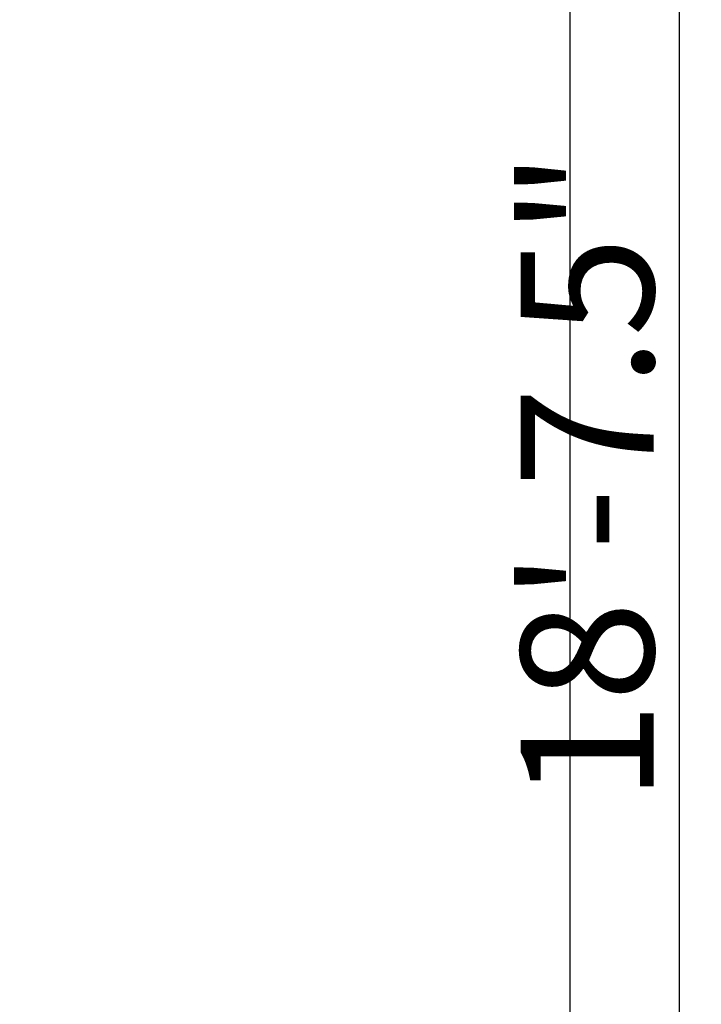
# Model space of a CAD drawing. Units: inches. Extents: x 2083 to 3317, y 1141 to 2115.
# Tile 245 of 256: x 3130 to 3191, y 1327 to 1416. Entities that reach past the tile are written whole.
import ezdxf

# ---------------------------------------------------------------- set-up
doc = ezdxf.new("R2010")
doc.units = ezdxf.units.IN
doc.layers.add('A-ANNO-DIMS', color=2, linetype='Continuous', lineweight=18)
doc.styles.get("Standard").update_dxf_attribs({"font": 'arial.ttf'})
doc.dimstyles.new('ISO-25', dxfattribs={"dimtxt": 12, "dimasz": 12, "dimexe": 1.25, "dimexo": 0.625, "dimtad": 1, "dimlunit": 3, "dimtxsty": 'Standard', "dimcen": 2.5, "dimadec": 0, "dimazin": 0, "dimtfac": 1, "dimtmove": 0, "dimatfit": 3, "dimfxl": 1, "dimarcsym": 0})

# ---------------------------------------------------------------- blocks, each defined once
blk = doc.blocks.new('*D9')
at = {"layer": 'A-ANNO-DIMS', "color": 0, "lineweight": -2, "transparency": 16777216}
for p, q in [((3127.585, 1486.761), (3190.403, 1486.761)), ((3189.153, 1474.761), (3189.153, 1275.261)), ((3127.585, 1263.261), (3190.403, 1263.261))]:
    blk.add_line(p, q, dxfattribs=at)
at = {"layer": 'A-ANNO-DIMS', "color": 0, "transparency": 16777216}
for points in [[(3187.153, 1474.761), (3191.153, 1474.761), (3189.153, 1486.761)], [(3187.153, 1275.261), (3191.153, 1275.261), (3189.153, 1263.261)]]:
    blk.add_solid(points, dxfattribs=at)
at = {"layer": 'Defpoints', "color": 0, "transparency": 16777216}
for p in [(3126.96, 1486.761), (3126.96, 1263.261), (3189.153, 1263.261)]:
    blk.add_point(p, dxfattribs=at)
at = {"layer": 'A-ANNO-DIMS', "color": 0, "transparency": 16777216, "insert": (3182.401, 1375.011), "char_height": 12, "attachment_point": 5, "rotation": 90}
blk.add_mtext('18\'-7.5"', dxfattribs=at)
blk = doc.blocks.new('*D35')
at = {"layer": 'A-ANNO-DIMS', "color": 0, "lineweight": -2, "transparency": 16777216}
for p, q in [((3127.585, 2020.761), (3180.56, 2020.761)), ((3179.31, 1275.261), (3179.31, 2008.761)), ((3127.585, 1263.261), (3180.56, 1263.261))]:
    blk.add_line(p, q, dxfattribs=at)
at = {"layer": 'A-ANNO-DIMS', "color": 0, "transparency": 16777216}
for points in [[(3177.31, 2008.761), (3181.31, 2008.761), (3179.31, 2020.761)], [(3177.31, 1275.261), (3181.31, 1275.261), (3179.31, 1263.261)]]:
    blk.add_solid(points, dxfattribs=at)
at = {"layer": 'Defpoints', "color": 0, "transparency": 16777216}
for p in [(3126.96, 2020.761), (3179.31, 2020.761), (3126.96, 1263.261)]:
    blk.add_point(p, dxfattribs=at)
at = {"layer": 'A-ANNO-DIMS', "color": 0, "transparency": 16777216, "insert": (3172.476, 1642.011), "char_height": 12, "attachment_point": 5, "rotation": 90}
blk.add_mtext('63\'-1 1/2"', dxfattribs=at)

msp = doc.modelspace()

# ---------------------------------------------------------------- dimensions: what is measured, and where the dimension line sits
at = {"layer": 'A-ANNO-DIMS'}
for base, p1, p2, override, picture, middle in [((3179.31, 2020.761), (3126.96, 1263.261), (3126.96, 2020.761), {"dimdec": 1, "dimlfac": 1, "dimrnd": 0, "dimzin": 1, "dimdsep": 46, "dimlunit": 4, "dimfrac": 2}, '*D35', (3172.476, 1642.011)), ((3189.153, 1263.261), (3126.96, 1486.761), (3126.96, 1263.261), {"dimclrd": 0, "dimclre": 0, "dimclrt": 0}, '*D9', (3182.401, 1375.011))]:
    dim = msp.add_linear_dim(base=base, p1=p1, p2=p2, angle=90, dimstyle='ISO-25', override=override, dxfattribs=at)
    dim.commit()
    dim.dimension.update_dxf_attribs({"geometry": picture, "text_midpoint": middle})

doc.saveas('drawing.dxf')
